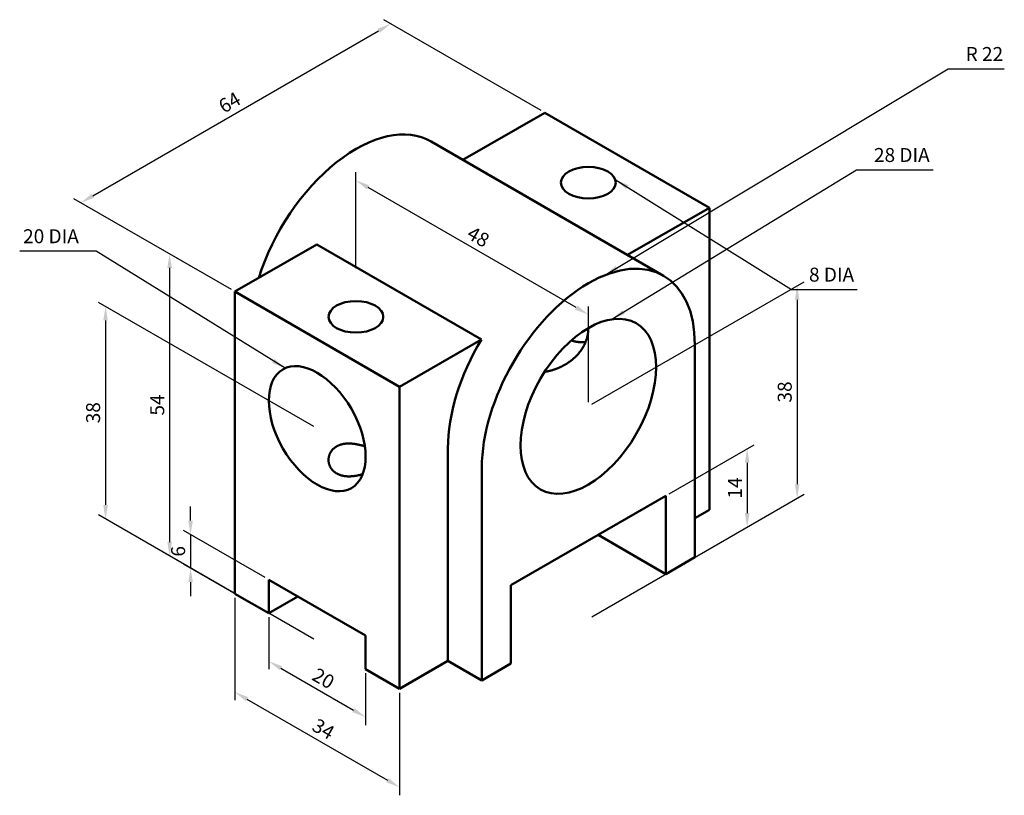
# Model space of a CAD drawing. Units: millimetres. Extents: x 2768 to 2945, y 1762 to 1900.
import ezdxf

# ---------------------------------------------------------------- set-up
doc = ezdxf.new("R2010")
doc.units = ezdxf.units.MM
for name, color, linetype, lineweight in [('M-DIMS', 2, 'Continuous', 25), ('M-OUTL', 7, 'Continuous', 50), ('M-TEXT', 7, 'Continuous', 25)]:
    doc.layers.add(name, color=color, linetype=linetype, lineweight=lineweight)
doc.styles.get("Standard").update_dxf_attribs({"font": 'arial.ttf'})
doc.dimstyles.new('ISO-25', dxfattribs={"dimtxt": 2.5, "dimasz": 2.5, "dimexe": 1.25, "dimexo": 0.625, "dimtad": 1, "dimtxsty": 'Standard', "dimcen": 2.5, "dimadec": 0, "dimazin": 0, "dimtfac": 1, "dimtmove": 0, "dimatfit": 3, "dimfxl": 1, "dimarcsym": 0})

# ---------------------------------------------------------------- blocks, each defined once
blk = doc.blocks.new('*D1')
at = {"layer": 'Defpoints', "color": 0, "transparency": 16777216}
for p in [(2812.95, 1794.22), (2830.27, 1784.22), (2830.27, 1775.64)]:
    blk.add_point(p, dxfattribs=at)
at = {"layer": 'M-DIMS', "color": 0, "lineweight": -2, "transparency": 16777216}
for p, q in [((2812.95, 1793.49), (2812.95, 1784.19)), ((2815.11, 1784.39), (2828.1, 1776.89)), ((2830.27, 1783.49), (2830.27, 1774.19))]:
    blk.add_line(p, q, dxfattribs=at)
at = {"layer": 'M-DIMS', "color": 0, "transparency": 16777216}
for points in [[(2815.32, 1784.75), (2814.91, 1784.03), (2812.95, 1785.64)], [(2828.31, 1777.25), (2827.9, 1776.53), (2830.27, 1775.64)]]:
    blk.add_solid(points, dxfattribs=at)
at = {"layer": 'M-DIMS', "color": 0, "transparency": 16777216, "insert": (2822.56, 1782.28), "char_height": 2.5, "attachment_point": 5, "rotation": 330}
blk.add_mtext('20', dxfattribs=at)
blk = doc.blocks.new('*D2')
at = {"layer": 'Defpoints', "color": 0, "transparency": 16777216}
for p in [(2806.89, 1797.72), (2836.33, 1780.72), (2836.33, 1763.11)]:
    blk.add_point(p, dxfattribs=at)
at = {"layer": 'M-DIMS', "color": 0, "lineweight": -2, "transparency": 16777216}
for p, q in [((2806.89, 1796.99), (2806.89, 1778.66)), ((2809.05, 1778.86), (2834.17, 1764.36)), ((2836.33, 1779.99), (2836.33, 1761.66))]:
    blk.add_line(p, q, dxfattribs=at)
at = {"layer": 'M-DIMS', "color": 0, "transparency": 16777216}
for points in [[(2809.26, 1779.22), (2808.84, 1778.5), (2806.89, 1780.11)], [(2834.38, 1764.72), (2833.96, 1764), (2836.33, 1763.11)]]:
    blk.add_solid(points, dxfattribs=at)
at = {"layer": 'M-DIMS', "color": 0, "transparency": 16777216, "insert": (2822.56, 1773.25), "char_height": 2.5, "attachment_point": 5, "rotation": 330}
blk.add_mtext('34', dxfattribs=at)
blk = doc.blocks.new('*D3')
at = {"layer": 'Defpoints', "color": 0, "transparency": 16777216}
for p in [(2798.96, 1802.29), (2812.95, 1800.22), (2812.95, 1794.22)]:
    blk.add_point(p, dxfattribs=at)
at = {"layer": 'M-DIMS', "color": 0, "lineweight": -2, "transparency": 16777216}
for p, q in [((2798.96, 1810.79), (2798.96, 1813.29)), ((2812.32, 1800.58), (2797.71, 1809.01)), ((2798.96, 1808.29), (2798.96, 1802.29)), ((2812.32, 1794.58), (2797.71, 1803.01)), ((2798.96, 1799.79), (2798.96, 1797.29))]:
    blk.add_line(p, q, dxfattribs=at)
at = {"layer": 'M-DIMS', "color": 0, "transparency": 16777216}
for points in [[(2798.55, 1810.79), (2799.38, 1810.79), (2798.96, 1808.29)], [(2798.55, 1799.79), (2799.38, 1799.79), (2798.96, 1802.29)]]:
    blk.add_solid(points, dxfattribs=at)
at = {"layer": 'M-DIMS', "color": 0, "transparency": 16777216, "insert": (2797.06, 1805.29), "char_height": 2.5, "attachment_point": 5, "rotation": 90}
blk.add_mtext('6', dxfattribs=at)
blk = doc.blocks.new('*D4')
at = {"layer": 'Defpoints', "color": 0, "transparency": 16777216}
for p in [(2821.61, 1827.22), (2783.75, 1811.07), (2821.61, 1789.22)]:
    blk.add_point(p, dxfattribs=at)
at = {"layer": 'M-DIMS', "color": 0, "lineweight": -2, "transparency": 16777216}
for p, q in [((2820.98, 1827.58), (2782.5, 1849.79)), ((2783.75, 1846.57), (2783.75, 1813.57)), ((2820.98, 1789.58), (2782.5, 1811.79))]:
    blk.add_line(p, q, dxfattribs=at)
at = {"layer": 'M-DIMS', "color": 0, "transparency": 16777216}
for points in [[(2783.34, 1846.57), (2784.17, 1846.57), (2783.75, 1849.07)], [(2783.34, 1813.57), (2784.17, 1813.57), (2783.75, 1811.07)]]:
    blk.add_solid(points, dxfattribs=at)
at = {"layer": 'M-DIMS', "color": 0, "transparency": 16777216, "insert": (2781.85, 1830.07), "char_height": 2.5, "attachment_point": 5, "rotation": 90}
blk.add_mtext('38', dxfattribs=at)
blk = doc.blocks.new('*D5')
at = {"layer": 'Defpoints', "color": 0, "transparency": 16777216}
for p in [(2806.89, 1851.72), (2795.21, 1804.45), (2806.89, 1797.72)]:
    blk.add_point(p, dxfattribs=at)
at = {"layer": 'M-DIMS', "color": 0, "lineweight": -2, "transparency": 16777216}
for p, q in [((2806.26, 1852.08), (2793.96, 1859.18)), ((2795.21, 1855.95), (2795.21, 1806.95)), ((2806.26, 1798.08), (2793.96, 1805.18))]:
    blk.add_line(p, q, dxfattribs=at)
at = {"layer": 'M-DIMS', "color": 0, "transparency": 16777216}
for points in [[(2794.8, 1855.95), (2795.63, 1855.95), (2795.21, 1858.45)], [(2794.8, 1806.95), (2795.63, 1806.95), (2795.21, 1804.45)]]:
    blk.add_solid(points, dxfattribs=at)
at = {"layer": 'M-DIMS', "color": 0, "transparency": 16777216, "insert": (2793.32, 1831.45), "char_height": 2.5, "attachment_point": 5, "rotation": 90}
blk.add_mtext('54', dxfattribs=at)
blk = doc.blocks.new('*D6')
at = {"layer": 'Defpoints', "color": 0, "transparency": 16777216}
for p in [(2834.76, 1899.62), (2862.31, 1883.72), (2806.89, 1851.72)]:
    blk.add_point(p, dxfattribs=at)
at = {"layer": 'M-DIMS', "color": 0, "lineweight": -2, "transparency": 16777216}
for p, q in [((2861.69, 1884.08), (2833.51, 1900.34)), ((2781.5, 1868.87), (2832.6, 1898.37)), ((2806.26, 1852.08), (2778.09, 1868.34))]:
    blk.add_line(p, q, dxfattribs=at)
at = {"layer": 'M-DIMS', "color": 0, "transparency": 16777216}
for points in [[(2832.39, 1898.73), (2832.81, 1898.01), (2834.76, 1899.62)], [(2781.29, 1869.23), (2781.71, 1868.51), (2779.34, 1867.62)]]:
    blk.add_solid(points, dxfattribs=at)
at = {"layer": 'M-DIMS', "color": 0, "transparency": 16777216, "insert": (2806.1, 1885.27), "char_height": 2.5, "attachment_point": 5, "rotation": 30}
blk.add_mtext('64', dxfattribs=at)
blk = doc.blocks.new('*D7')
at = {"layer": 'Defpoints', "color": 0, "transparency": 16777216}
for p in [(2870.11, 1831.22), (2907.46, 1814.78), (2870.11, 1793.22)]:
    blk.add_point(p, dxfattribs=at)
at = {"layer": 'M-DIMS', "color": 0, "lineweight": -2, "transparency": 16777216}
for p, q in [((2870.73, 1831.58), (2908.71, 1853.5)), ((2907.46, 1850.28), (2907.46, 1817.28)), ((2870.73, 1793.58), (2908.71, 1815.5))]:
    blk.add_line(p, q, dxfattribs=at)
at = {"layer": 'M-DIMS', "color": 0, "transparency": 16777216}
for points in [[(2907.04, 1850.28), (2907.87, 1850.28), (2907.46, 1852.78)], [(2907.04, 1817.28), (2907.87, 1817.28), (2907.46, 1814.78)]]:
    blk.add_solid(points, dxfattribs=at)
at = {"layer": 'M-DIMS', "color": 0, "transparency": 16777216, "insert": (2905.56, 1833.78), "char_height": 2.5, "attachment_point": 5, "rotation": 90}
blk.add_mtext('38', dxfattribs=at)
blk = doc.blocks.new('*D8')
at = {"layer": 'Defpoints', "color": 0, "transparency": 16777216}
for p in [(2883.96, 1815.22), (2898.52, 1809.62), (2883.96, 1801.22)]:
    blk.add_point(p, dxfattribs=at)
at = {"layer": 'M-DIMS', "color": 0, "lineweight": -2, "transparency": 16777216}
for p, q in [((2884.59, 1815.58), (2899.77, 1824.34)), ((2898.52, 1821.12), (2898.52, 1812.12)), ((2884.59, 1801.58), (2899.77, 1810.34))]:
    blk.add_line(p, q, dxfattribs=at)
at = {"layer": 'M-DIMS', "color": 0, "transparency": 16777216}
for points in [[(2898.1, 1821.12), (2898.94, 1821.12), (2898.52, 1823.62)], [(2898.1, 1812.12), (2898.94, 1812.12), (2898.52, 1809.62)]]:
    blk.add_solid(points, dxfattribs=at)
at = {"layer": 'M-DIMS', "color": 0, "transparency": 16777216, "insert": (2896.64, 1816.62), "char_height": 2.5, "attachment_point": 5, "rotation": 90}
blk.add_mtext('14', dxfattribs=at)
blk = doc.blocks.new('*D9')
at = {"layer": 'Defpoints', "color": 0, "transparency": 16777216}
for p in [(2828.54, 1871.61), (2828.54, 1855.22), (2870.11, 1831.22)]:
    blk.add_point(p, dxfattribs=at)
at = {"layer": 'M-DIMS', "color": 0, "lineweight": -2, "transparency": 16777216}
for p, q in [((2828.54, 1855.94), (2828.54, 1873.06)), ((2867.94, 1848.86), (2830.7, 1870.36)), ((2870.11, 1831.94), (2870.11, 1849.06))]:
    blk.add_line(p, q, dxfattribs=at)
at = {"layer": 'M-DIMS', "color": 0, "transparency": 16777216}
for points in [[(2830.91, 1870.73), (2830.49, 1870), (2828.54, 1871.61)], [(2868.15, 1849.23), (2867.73, 1848.5), (2870.11, 1847.61)]]:
    blk.add_solid(points, dxfattribs=at)
at = {"layer": 'M-DIMS', "color": 0, "transparency": 16777216, "insert": (2850.27, 1861.26), "char_height": 2.5, "attachment_point": 5, "rotation": 330}
blk.add_mtext('48', dxfattribs=at)

msp = doc.modelspace()

# ---------------------------------------------------------------- linework, layer by layer
at = {"layer": 'M-OUTL'}
for p, q in [((2847.688, 1875.272), (2862.313, 1883.715)), ((2862.313, 1883.715), (2891.758, 1866.715)), ((2842.01, 1878.55), (2883.579, 1854.55)), ((2891.758, 1866.715), (2877.133, 1858.272)), ((2891.758, 1866.715), (2891.758, 1812.715)), ((2821.523, 1860.165), (2806.887, 1851.715)), ((2850.968, 1843.165), (2821.523, 1860.165)), ((2806.887, 1851.715), (2806.887, 1797.715)), ((2836.332, 1834.715), (2806.887, 1851.715)), ((2836.332, 1834.715), (2850.968, 1843.165)), ((2889.16, 1842.215), (2889.16, 1804.215)), ((2836.332, 1780.715), (2836.332, 1834.715)), ((2844.992, 1823.715), (2844.992, 1785.715)), ((2851.055, 1820.215), (2851.055, 1782.215)), ((2883.964, 1815.215), (2856.251, 1799.215)), ((2883.964, 1801.215), (2883.964, 1815.215)), ((2891.758, 1812.715), (2889.16, 1811.215)), ((2883.964, 1801.215), (2871.839, 1808.215)), ((2889.16, 1804.215), (2883.964, 1801.215)), ((2812.949, 1794.215), (2812.949, 1800.215)), ((2812.949, 1800.215), (2830.27, 1790.215)), ((2856.251, 1799.215), (2856.251, 1785.215)), ((2806.887, 1797.715), (2812.949, 1794.215)), ((2812.949, 1794.215), (2818.146, 1797.215)), ((2830.27, 1790.215), (2830.27, 1784.215)), ((2830.27, 1784.215), (2836.332, 1780.715)), ((2844.992, 1785.715), (2836.332, 1780.715)), ((2844.992, 1785.715), (2851.055, 1782.215)), ((2856.251, 1785.215), (2851.055, 1782.215))]:
    msp.add_line(p, q, dxfattribs=at)
for points in [[(2870.107, 1845.215), (2870.107, 1845.122), (2870.105, 1845.028), (2870.101, 1844.934), (2870.097, 1844.841), (2870.091, 1844.748), (2870.084, 1844.655), (2870.075, 1844.563), (2870.066, 1844.471), (2870.055, 1844.379), (2870.042, 1844.287), (2870.029, 1844.196), (2870.014, 1844.105), (2869.998, 1844.014), (2869.981, 1843.924), (2869.962, 1843.835), (2869.943, 1843.746), (2869.922, 1843.657), (2869.9, 1843.569), (2869.877, 1843.481), (2869.852, 1843.394), (2869.827, 1843.307), (2869.801, 1843.221), (2869.773, 1843.136), (2869.744, 1843.051), (2869.715, 1842.967), (2869.684, 1842.883), (2869.653, 1842.8), (2869.62, 1842.718), (2869.586, 1842.636), (2869.552, 1842.555), (2869.516, 1842.474), (2869.48, 1842.395), (2869.442, 1842.315), (2869.404, 1842.237), (2869.365, 1842.159), (2869.325, 1842.081), (2869.284, 1842.005), (2869.242, 1841.929), (2869.2, 1841.854), (2869.157, 1841.779), (2869.113, 1841.705), (2869.068, 1841.632), (2869.023, 1841.56), (2868.977, 1841.488), (2868.93, 1841.417), (2868.882, 1841.346), (2868.834, 1841.277), (2868.786, 1841.208), (2868.736, 1841.139), (2868.686, 1841.072), (2868.636, 1841.005), (2868.584, 1840.938), (2868.533, 1840.873), (2868.48, 1840.808), (2868.427, 1840.743), (2868.374, 1840.68), (2868.32, 1840.617), (2868.265, 1840.554), (2868.21, 1840.493), (2868.155, 1840.432), (2868.099, 1840.371), (2868.043, 1840.312), (2867.986, 1840.253), (2867.928, 1840.194), (2867.871, 1840.137), (2867.812, 1840.079), (2867.754, 1840.023), (2867.695, 1839.967), (2867.635, 1839.912), (2867.576, 1839.857), (2867.515, 1839.803), (2867.455, 1839.75), (2867.394, 1839.697), (2867.333, 1839.645), (2867.271, 1839.594), (2867.209, 1839.543), (2867.147, 1839.493), (2867.084, 1839.443), (2867.021, 1839.394), (2866.958, 1839.346), (2866.894, 1839.298), (2866.831, 1839.25), (2866.767, 1839.204), (2866.702, 1839.158), (2866.638, 1839.112), (2866.573, 1839.067), (2866.507, 1839.023), (2866.442, 1838.979), (2866.376, 1838.936), (2866.31, 1838.894), (2866.244, 1838.852), (2866.178, 1838.81), (2866.111, 1838.769), (2866.045, 1838.729), (2865.978, 1838.689), (2865.911, 1838.65)], [(2867.063, 1843.01), (2867.088, 1842.999), (2867.113, 1842.99), (2867.138, 1842.98), (2867.163, 1842.97), (2867.189, 1842.961), (2867.214, 1842.951), (2867.24, 1842.942), (2867.265, 1842.933), (2867.291, 1842.925), (2867.316, 1842.916), (2867.342, 1842.908), (2867.368, 1842.899), (2867.394, 1842.891), (2867.42, 1842.883), (2867.446, 1842.876), (2867.472, 1842.868), (2867.498, 1842.861), (2867.525, 1842.854), (2867.551, 1842.846), (2867.577, 1842.84), (2867.604, 1842.833), (2867.63, 1842.826), (2867.657, 1842.82), (2867.683, 1842.814), (2867.71, 1842.807), (2867.737, 1842.801), (2867.763, 1842.796), (2867.79, 1842.79), (2867.817, 1842.785), (2867.844, 1842.779), (2867.871, 1842.774), (2867.897, 1842.769), (2867.924, 1842.764), (2867.951, 1842.76), (2867.978, 1842.755), (2868.005, 1842.751), (2868.032, 1842.747), (2868.059, 1842.742), (2868.087, 1842.739), (2868.114, 1842.735), (2868.141, 1842.731), (2868.168, 1842.728), (2868.195, 1842.724), (2868.222, 1842.721), (2868.25, 1842.718), (2868.277, 1842.715), (2868.304, 1842.712), (2868.331, 1842.71), (2868.358, 1842.707), (2868.386, 1842.705), (2868.413, 1842.703), (2868.44, 1842.701), (2868.467, 1842.699), (2868.495, 1842.697), (2868.522, 1842.695), (2868.549, 1842.694), (2868.576, 1842.692), (2868.603, 1842.691), (2868.631, 1842.69), (2868.658, 1842.689), (2868.685, 1842.688), (2868.712, 1842.687), (2868.739, 1842.687), (2868.766, 1842.686), (2868.793, 1842.686), (2868.821, 1842.685), (2868.848, 1842.685), (2868.875, 1842.685), (2868.902, 1842.685), (2868.929, 1842.685), (2868.956, 1842.686), (2868.983, 1842.686), (2869.01, 1842.687), (2869.037, 1842.687), (2869.064, 1842.688), (2869.091, 1842.689), (2869.118, 1842.69), (2869.145, 1842.691), (2869.171, 1842.692), (2869.198, 1842.693), (2869.225, 1842.695), (2869.252, 1842.696), (2869.279, 1842.698), (2869.305, 1842.7), (2869.332, 1842.701), (2869.359, 1842.703), (2869.385, 1842.705), (2869.412, 1842.707), (2869.439, 1842.71), (2869.465, 1842.712), (2869.492, 1842.714), (2869.518, 1842.717), (2869.545, 1842.719), (2869.571, 1842.722), (2869.597, 1842.725), (2869.624, 1842.727)], [(2865.911, 1838.65), (2865.874, 1838.629), (2865.838, 1838.609), (2865.802, 1838.588), (2865.765, 1838.568), (2865.729, 1838.548), (2865.692, 1838.528), (2865.656, 1838.508), (2865.619, 1838.488), (2865.583, 1838.469), (2865.546, 1838.45), (2865.509, 1838.43), (2865.473, 1838.411), (2865.436, 1838.392), (2865.399, 1838.374), (2865.362, 1838.355), (2865.325, 1838.337), (2865.288, 1838.319), (2865.251, 1838.301), (2865.214, 1838.283), (2865.177, 1838.265), (2865.14, 1838.247), (2865.102, 1838.23), (2865.065, 1838.213), (2865.028, 1838.196), (2864.99, 1838.179), (2864.953, 1838.162), (2864.916, 1838.145), (2864.878, 1838.129), (2864.841, 1838.112), (2864.803, 1838.096), (2864.766, 1838.08), (2864.728, 1838.064), (2864.69, 1838.049), (2864.653, 1838.033), (2864.615, 1838.018), (2864.577, 1838.003), (2864.54, 1837.988), (2864.502, 1837.973), (2864.464, 1837.958), (2864.426, 1837.943), (2864.388, 1837.929), (2864.35, 1837.915), (2864.312, 1837.901), (2864.274, 1837.887), (2864.236, 1837.873), (2864.198, 1837.859), (2864.16, 1837.846), (2864.122, 1837.833), (2864.084, 1837.819), (2864.046, 1837.806), (2864.008, 1837.794), (2863.969, 1837.781), (2863.931, 1837.768), (2863.893, 1837.756), (2863.855, 1837.744), (2863.816, 1837.732), (2863.778, 1837.72), (2863.74, 1837.708), (2863.701, 1837.696), (2863.663, 1837.685), (2863.625, 1837.674), (2863.586, 1837.663), (2863.548, 1837.652), (2863.509, 1837.641), (2863.471, 1837.63), (2863.433, 1837.62), (2863.394, 1837.61), (2863.356, 1837.599), (2863.317, 1837.589), (2863.279, 1837.58), (2863.24, 1837.57), (2863.202, 1837.561), (2863.163, 1837.551), (2863.124, 1837.542), (2863.086, 1837.533), (2863.047, 1837.524), (2863.009, 1837.515), (2862.97, 1837.507), (2862.932, 1837.499), (2862.893, 1837.49), (2862.854, 1837.482), (2862.816, 1837.474), (2862.777, 1837.467), (2862.739, 1837.459), (2862.7, 1837.452), (2862.662, 1837.445), (2862.623, 1837.438), (2862.584, 1837.431), (2862.546, 1837.424), (2862.507, 1837.417), (2862.469, 1837.411), (2862.43, 1837.405), (2862.392, 1837.399), (2862.353, 1837.393), (2862.314, 1837.387), (2862.276, 1837.382)], [(2830.136, 1824.043), (2830.027, 1824.08), (2829.919, 1824.114), (2829.81, 1824.148), (2829.702, 1824.18), (2829.594, 1824.212), (2829.487, 1824.241), (2829.379, 1824.27), (2829.273, 1824.297), (2829.166, 1824.323), (2829.061, 1824.348), (2828.955, 1824.371), (2828.851, 1824.393), (2828.747, 1824.414), (2828.644, 1824.433), (2828.541, 1824.452), (2828.439, 1824.468), (2828.337, 1824.484), (2828.237, 1824.498), (2828.136, 1824.511), (2828.037, 1824.522), (2827.938, 1824.533), (2827.84, 1824.542), (2827.743, 1824.549), (2827.647, 1824.555), (2827.551, 1824.56), (2827.456, 1824.564), (2827.362, 1824.566), (2827.269, 1824.567), (2827.176, 1824.566), (2827.085, 1824.564), (2826.994, 1824.561), (2826.904, 1824.556), (2826.815, 1824.55), (2826.727, 1824.543), (2826.64, 1824.534), (2826.554, 1824.524), (2826.469, 1824.512), (2826.384, 1824.499), (2826.301, 1824.485), (2826.219, 1824.469), (2826.137, 1824.452), (2826.057, 1824.434), (2825.977, 1824.414), (2825.899, 1824.393), (2825.821, 1824.37), (2825.745, 1824.346), (2825.67, 1824.321), (2825.596, 1824.294), (2825.522, 1824.266), (2825.45, 1824.237), (2825.379, 1824.206), (2825.31, 1824.174), (2825.241, 1824.14), (2825.174, 1824.105), (2825.107, 1824.069), (2825.042, 1824.032), (2824.979, 1823.993), (2824.916, 1823.953), (2824.855, 1823.911), (2824.795, 1823.869), (2824.736, 1823.825), (2824.679, 1823.779), (2824.623, 1823.733), (2824.568, 1823.685), (2824.514, 1823.636), (2824.463, 1823.586), (2824.412, 1823.535), (2824.363, 1823.483), (2824.315, 1823.429), (2824.269, 1823.374), (2824.224, 1823.319), (2824.181, 1823.262), (2824.139, 1823.204), (2824.099, 1823.145), (2824.06, 1823.085), (2824.022, 1823.024), (2823.987, 1822.962), (2823.953, 1822.899), (2823.92, 1822.834), (2823.889, 1822.77), (2823.86, 1822.704), (2823.833, 1822.637), (2823.807, 1822.569), (2823.783, 1822.501), (2823.76, 1822.431), (2823.74, 1822.361), (2823.721, 1822.291), (2823.704, 1822.219), (2823.689, 1822.147), (2823.676, 1822.074), (2823.665, 1822), (2823.656, 1821.926), (2823.648, 1821.851), (2823.643, 1821.776), (2823.64, 1821.7), (2823.639, 1821.624)], [(2823.639, 1821.624), (2823.64, 1821.561), (2823.642, 1821.498), (2823.646, 1821.435), (2823.651, 1821.371), (2823.657, 1821.307), (2823.666, 1821.243), (2823.675, 1821.179), (2823.687, 1821.115), (2823.7, 1821.051), (2823.715, 1820.986), (2823.731, 1820.922), (2823.749, 1820.857), (2823.769, 1820.793), (2823.79, 1820.728), (2823.814, 1820.664), (2823.839, 1820.6), (2823.866, 1820.536), (2823.895, 1820.472), (2823.926, 1820.408), (2823.959, 1820.345), (2823.994, 1820.282), (2824.031, 1820.219), (2824.069, 1820.157), (2824.11, 1820.096), (2824.153, 1820.035), (2824.198, 1819.975), (2824.245, 1819.915), (2824.294, 1819.857), (2824.345, 1819.799), (2824.398, 1819.742), (2824.453, 1819.686), (2824.51, 1819.631), (2824.57, 1819.577), (2824.631, 1819.524), (2824.694, 1819.473), (2824.759, 1819.422), (2824.826, 1819.374), (2824.895, 1819.326), (2824.965, 1819.281), (2825.038, 1819.237), (2825.111, 1819.194), (2825.187, 1819.153), (2825.263, 1819.114), (2825.341, 1819.076), (2825.421, 1819.041), (2825.501, 1819.007), (2825.583, 1818.974), (2825.666, 1818.944), (2825.75, 1818.915), (2825.834, 1818.889), (2825.919, 1818.863), (2826.005, 1818.84), (2826.092, 1818.819), (2826.179, 1818.799), (2826.266, 1818.781), (2826.354, 1818.765), (2826.442, 1818.75), (2826.531, 1818.737), (2826.62, 1818.725), (2826.708, 1818.715), (2826.797, 1818.707), (2826.886, 1818.7), (2826.975, 1818.694), (2827.064, 1818.69), (2827.153, 1818.687), (2827.241, 1818.685), (2827.33, 1818.685), (2827.418, 1818.686), (2827.506, 1818.688), (2827.594, 1818.692), (2827.682, 1818.696), (2827.769, 1818.702), (2827.856, 1818.708), (2827.943, 1818.716), (2828.029, 1818.725), (2828.115, 1818.734), (2828.201, 1818.745), (2828.286, 1818.756), (2828.371, 1818.768), (2828.455, 1818.781), (2828.539, 1818.795), (2828.623, 1818.81), (2828.706, 1818.825), (2828.788, 1818.842), (2828.87, 1818.858), (2828.952, 1818.876), (2829.033, 1818.894), (2829.114, 1818.913), (2829.195, 1818.932), (2829.274, 1818.952), (2829.354, 1818.973), (2829.432, 1818.994), (2829.511, 1819.015), (2829.589, 1819.037), (2829.666, 1819.06), (2829.742, 1819.083)]]:
    msp.add_lwpolyline(points, dxfattribs=at)
for centre, start_param, end_param in [((2828.538, 1855.215), 3.1415927, 5.0763296), ((2870.107, 1831.215), 2.3561945, 5.4977871), ((2864.045, 1834.715), 4.6834472, 5.4977871)]:
    msp.add_ellipse(centre, major_axis=(-13.472, -23.335), ratio=0.5773503, start_param=start_param, end_param=end_param, dxfattribs=at)
for centre, major_axis in [((2870.107, 1871.215), (-4.899, 0)), ((2828.538, 1847.215), (-4.899, 0)), ((2870.107, 1831.215), (-8.573, -14.849)), ((2821.61, 1827.215), (6.124, -10.607))]:
    msp.add_ellipse(centre, major_axis=major_axis, ratio=0.5773503, dxfattribs=at)

# ---------------------------------------------------------------- texts
at = {"layer": 'M-TEXT', "char_height": 2.5}
for s, insert, attachment_point in [('R 22', (2937.593, 1892.177), 7), ('28 DIA', (2921.198, 1874.121), 7), ('20 DIA', (2778.974, 1859.592), 9), ('8 DIA', (2909.573, 1852.729), 7)]:
    msp.add_mtext(s, dxfattribs=dict(at, insert=insert, attachment_point=attachment_point))

# ---------------------------------------------------------------- dimensions: what is measured, and where the dimension line sits
at = {"layer": 'M-DIMS'}
for p1, p2, distance, picture, middle in [((2806.887, 1851.715), (2862.313, 1883.715), 27.551, '*D6', (2806.099, 1885.268)), ((2870.107, 1831.215), (2828.538, 1855.215), -14.202, '*D9', (2850.273, 1861.262)), ((2806.887, 1851.715), (2806.887, 1797.715), -11.673, '*D5', (2793.318, 1831.455)), ((2870.107, 1831.215), (2870.107, 1793.215), 37.351, '*D7', (2905.555, 1833.78)), ((2821.61, 1827.215), (2821.61, 1789.215), -37.855, '*D4', (2781.852, 1830.071)), ((2883.964, 1815.215), (2883.964, 1801.215), 14.555, '*D8', (2896.638, 1816.619)), ((2812.949, 1800.215), (2812.949, 1794.215), -13.985, '*D3', (2797.063, 1805.29)), ((2806.887, 1797.715), (2836.332, 1780.715), -15.25, '*D2', (2822.561, 1773.254)), ((2812.949, 1794.215), (2830.27, 1784.215), -7.428, '*D1', (2822.56, 1782.285))]:
    dim = msp.add_aligned_dim(p1=p1, p2=p2, distance=distance, dimstyle='ISO-25', override={"dimclrd": 0, "dimclre": 0, "dimclrt": 0}, dxfattribs=at)
    dim.commit()
    dim.dimension.update_dxf_attribs({"geometry": picture, "text_midpoint": middle})

# ---------------------------------------------------------------- leaders
at = {"layer": 'M-DIMS', "annotation_type": 0, "has_hookline": 1}
for points, hookline_direction, text_width in [([(2873.054, 1854.652), (2934.468, 1891.552), (2936.968, 1891.552)], 0, 6.918), ([(2874.282, 1846.769), (2918.073, 1873.496), (2920.573, 1873.496)], 0, 10.58), ([(2874.917, 1871.752), (2906.448, 1852.104), (2908.948, 1852.104)], 0, 8.598), ([(2815.878, 1838.021), (2782.099, 1858.967), (2779.599, 1858.967)], 1, 10.58)]:
    msp.add_leader(points, dimstyle='ISO-25', dxfattribs=dict(at, hookline_direction=hookline_direction, text_width=text_width))

doc.saveas('drawing.dxf')
